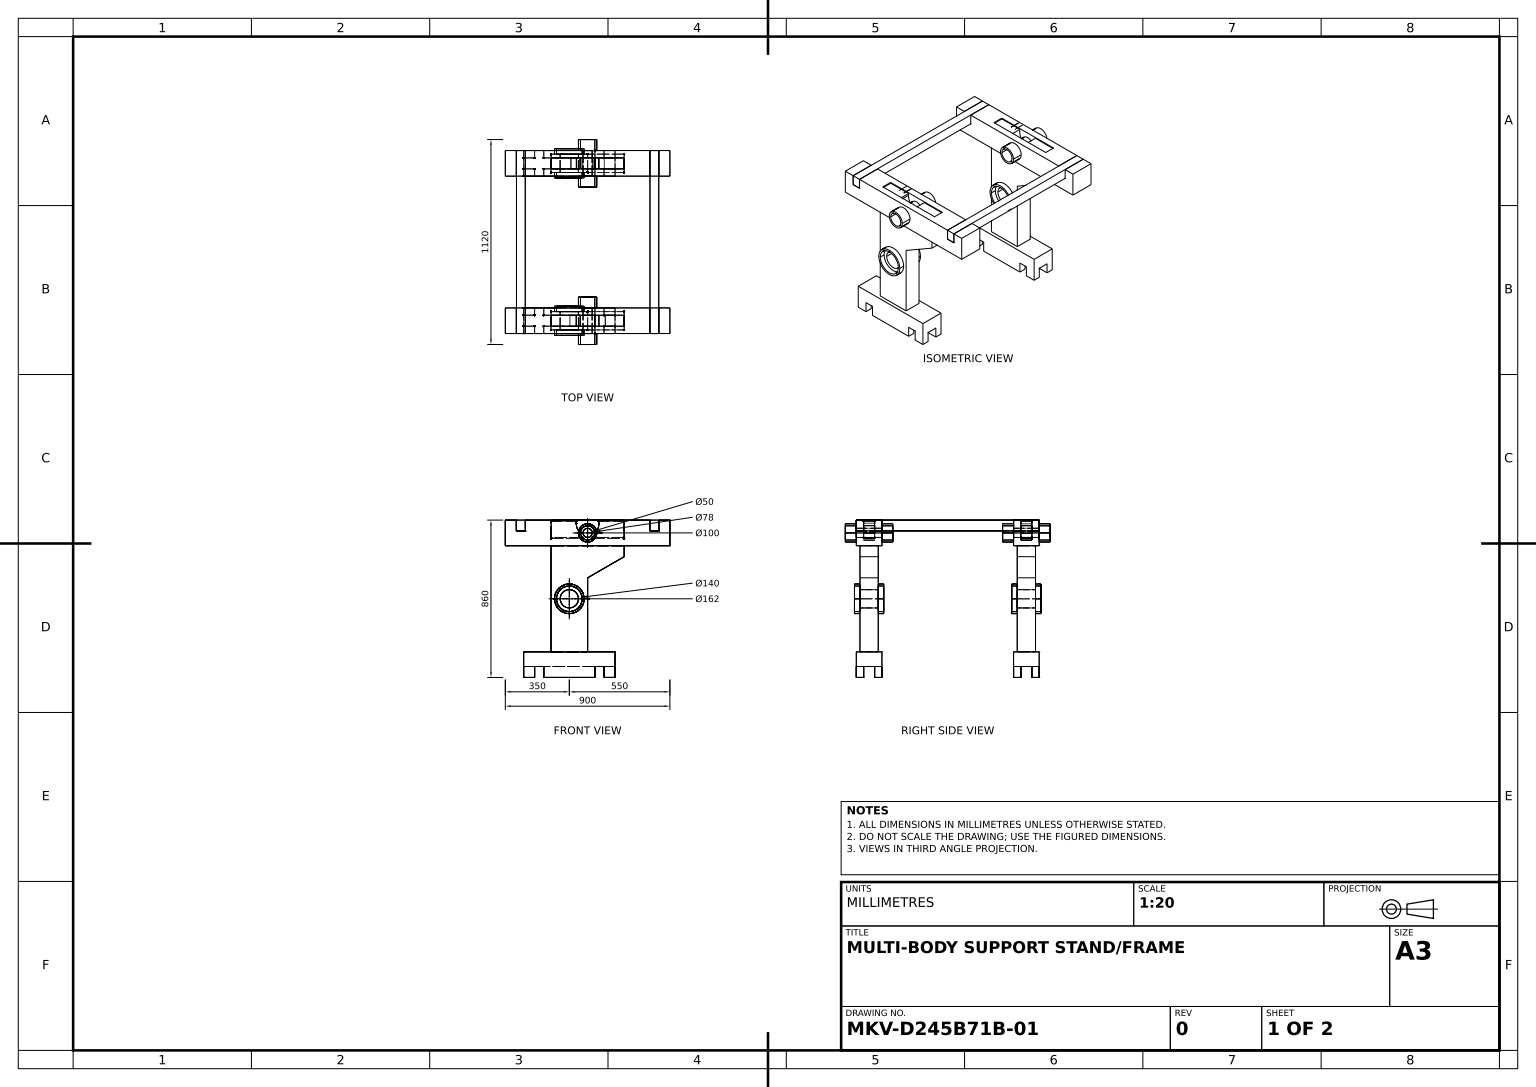
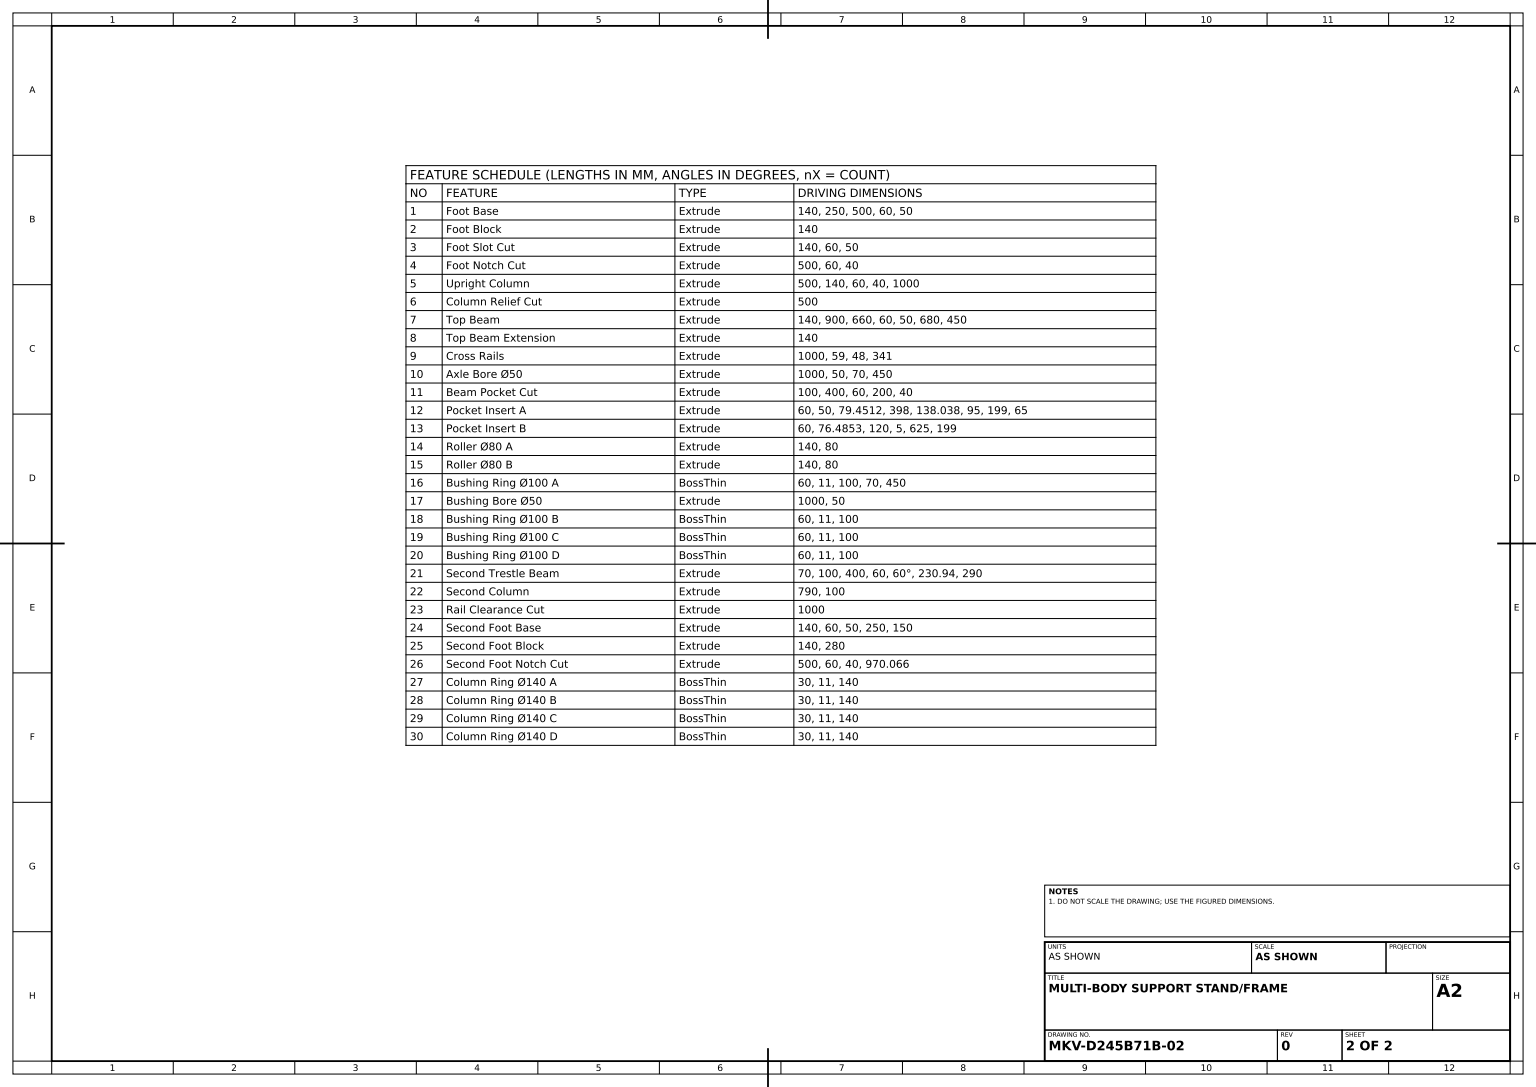
SolidWorks part; units mm, degrees
material "Plain Carbon Steel"
ref_plane "Front Plane" through (0, 0, 0) normal (0, 0, 1) x (1, 0, 0)
ref_plane "Top Plane" through (0, 0, 0) normal (0, 1, 0) x (1, 0, 0)
ref_plane "Right Plane" through (0, 0, 0) normal (1, 0, 0) x (0, 0, -1)
sketch "Foot Base Sketch" plane through (0, 0, 0) normal (0, 1, 0) x (1, 0, 0)
  line L0 (-250, 0) -> (-250, 140)
  line L1 (-250, 0) -> (250, 0)
  line L2 (-250, 140) -> (-190, 140)
  line L3 (-190, 140) -> (-190, 80)
  line L4 (-190, 80) -> (-140, 80)
  line L5 (-140, 80) -> (-140, 140)
  line L6 (-140, 140) -> (140, 140)
  line L7 (140, 140) -> (140, 80)
  line L8 (140, 80) -> (190, 80)
  line L9 (190, 80) -> (190, 140)
  line L10 (190, 140) -> (250, 140)
  line L11 (250, 140) -> (250, 0)
  dimension "D1" = 250
  dimension "D2" = 500
  dimension "D3" = 140
  dimension "D4" = 140
  dimension "D5" = 60
  dimension "D6" = 60
  dimension "D7" = 60
  dimension "D8" = 60
  dimension "D9" = 50
  dimension "D10" = 50
  dimension "D11" = 60
extrude "Foot Base" add sketch "Foot Base Sketch" along normal blind 140
sketch "Foot Block Sketch" plane through (0, 0, 0) normal (0, 0, 1) x (1, 0, 0)
  line L1 (-250, 140) -> (250, 140)
  line L2 (-250, 140) -> (-250, 0)
  line L3 (-250, 0) -> (250, 0)
  line L4 (250, 140) -> (250, 0)
extrude "Foot Block" add sketch "Foot Block Sketch" against normal blind 140
sketch "Foot Slot Sketch" plane through (0, 0, 0) normal (0, 0, 1) x (1, 0, 0)
  line L1 (-250, 0) -> (250, 0) construction
  line L2 (-190, 0) -> (-190, 60)
  line L3 (-190, 60) -> (-140, 60)
  line L4 (-140, 60) -> (-140, 0)
  line L6 (140, 0) -> (140, 60)
  line L7 (140, 60) -> (190, 60)
  line L8 (190, 60) -> (190, 0)
  line L13 (-190, 0) -> (-140, 0)
  line L14 (140, 0) -> (190, 0)
  line L15 (-250, 140) -> (-250, 0) construction
  line L16 (250, 140) -> (250, 0) construction
  point P17 (165, 60)
  dimension "D1" = 60
  dimension "D2" = 50
  dimension "D3" = 60
  dimension "D4" = 50
  dimension "D5" = 60
  dimension "D6" = 60
extrude "Foot Slot Cut" cut sketch "Foot Slot Sketch" against normal blind 140
sketch "Foot Notch Sketch" plane through (-250, 0, 0) normal (-1, 0, 0) x (0, 0, 1)
  line L0 (0, 140) -> (0, 0) construction
  line L3 (-140, 0) -> (0, 0) construction
  line L4 (-100, 0) -> (-100, 60)
  line L5 (-100, 60) -> (-40, 60)
  line L6 (-40, 60) -> (-40, 0)
  line L7 (-40, 0) -> (-100, 0)
  dimension "D1" = 60
  dimension "D2" = 60
  dimension "D3" = 40
extrude "Foot Notch Cut" cut sketch "Foot Notch Sketch" against normal blind 500
sketch "Upright Column Sketch" plane through (-250, 0, 0) normal (-1, 0, 0) x (0, 0, 1)
  line L0 (720, 140) -> (860, 140)
  line L1 (860, 140) -> (860, 0)
  line L2 (860, 0) -> (820, 0)
  line L3 (720, 0) -> (720, 140)
  line L4 (720, 0) -> (760, 0)
  line L5 (760, 0) -> (760, 60)
  line L6 (760, 60) -> (820, 60)
  line L7 (820, 60) -> (820, 0)
  line L8 (760, 0) -> (720, 0)
  line L9 (-140, 140) -> (-140, 0) construction
  dimension "D1" = 140
  dimension "D2" = 60
  dimension "D3" = 40
  dimension "D4" = 1000
  dimension "D5" = 60
extrude "Upright Column" add sketch "Upright Column Sketch" against normal blind 500 separate body contours L6 L7 L2 L1 L0 L3 L4 L5
sketch "Column Relief Sketch" plane through (0, 0, 720) normal (0, 0, -1) x (-1, 0, 0)
  line L0 (-190, 0) -> (-190, 60)
  line L1 (-190, 60) -> (-140, 60)
  line L2 (-190, 60) -> (-140, 60) construction
  line L3 (-140, 60) -> (-140, 0)
  line L4 (-140, 0) -> (-190, 0)
  line L5 (140, 60) -> (190, 60)
  line L6 (190, 60) -> (190, 0)
  line L7 (190, 0) -> (250, 0) construction
  line L8 (190, 60) -> (190, 0) construction
  line L9 (190, 0) -> (140, 0)
  line L10 (-140, 0) -> (140, 0) construction
  line L11 (-250, 0) -> (250, 0) construction
  line L12 (140, 0) -> (140, 60)
extrude "Column Relief Cut" cut sketch "Column Relief Sketch" against normal blind 500
sketch "Top Beam Sketch" plane through (0, 0, 860) normal (0, 0, 1) x (1, 0, 0)
  line L0 (-190, 60) -> (-140, 60) construction
  line L1 (450, 720) -> (-450, 720)
  line L2 (-450, 720) -> (-450, 860)
  line L3 (-450, 860) -> (-390, 860)
  line L4 (-390, 860) -> (-390, 800)
  line L5 (-390, 800) -> (-340, 800)
  line L6 (-340, 800) -> (-340, 860)
  line L9 (450, 720) -> (450, 860)
  line L10 (450, 860) -> (390, 860)
  line L11 (390, 860) -> (390, 800)
  line L12 (390, 800) -> (340, 800)
  line L13 (340, 800) -> (340, 860)
  line L14 (340, 860) -> (-340, 860)
  dimension "D1" = 900
  dimension "D2" = 660
  dimension "D3" = 140
  dimension "D4" = 60
  dimension "D5" = 50
  dimension "D6" = 60
  dimension "D7" = 680
  dimension "D8" = 140
  dimension "D9" = 60
  dimension "D10" = 60
  dimension "D11" = 60
  dimension "D12" = 450
extrude "Top Beam" add sketch "Top Beam Sketch" against normal blind 140 separate body
sketch "Top Beam Extension Sketch" plane through (0, 0, -140) normal (0, 0, -1) x (-1, 0, 0)
  line L0 (-450, 860) -> (-450, 720)
  line L1 (-450, 720) -> (450, 720)
  line L2 (450, 720) -> (450, 860)
  line L3 (450, 860) -> (390, 860)
  line L4 (390, 860) -> (390, 800)
  line L5 (390, 800) -> (340, 800)
  line L6 (340, 800) -> (340, 860)
  line L7 (340, 860) -> (-340, 860)
  line L8 (-340, 860) -> (-340, 800)
  line L9 (-340, 800) -> (-390, 800)
  line L10 (-390, 800) -> (-390, 860)
  line L11 (-390, 860) -> (-450, 860)
extrude "Top Beam Extension" add sketch "Top Beam Extension Sketch" against normal blind 140 separate body
sketch "Cross Rails Sketch" plane through (0, 0, 860) normal (0, 0, 1) x (1, 0, 0)
  line L1 (341, 860) -> (341, 801)
  line L3 (389, 860) -> (341, 860)
  line L4 (341, 801) -> (389, 801)
  line L5 (389, 801) -> (389, 860)
  line L7 (0, 860) -> (0, 140)
  line L8 (340, 860) -> (-340, 860) construction
  line L9 (250, 140) -> (-250, 140) construction
  line L10 (-389, 801) -> (-389, 860)
  line L11 (-341, 801) -> (-389, 801)
  line L12 (-341, 860) -> (-341, 801)
  line L13 (-389, 860) -> (-341, 860)
  dimension "D1" = 59
  dimension "D2" = 48
  dimension "D3" = 341
extrude "Cross Rails" add sketch "Cross Rails Sketch" against normal blind 1000 separate body contours L13 L10 L11 L12 | L4 L5 L3 L1
sketch "Axle Bore Ø50 Sketch" plane through (0, 0, 860) normal (0, 0, 1) x (1, 0, 0)
  line L0 (340, 860) -> (-340, 860) construction
  line L1 (450, 720) -> (450, 860) construction
  circle A0 centre (0, 790) radius 25
  dimension "D1" = 50
  dimension "D2" = 70
  dimension "D3" = 450
extrude "Axle Bore Ø50" cut sketch "Axle Bore Ø50 Sketch" against normal blind 1000
sketch "Beam Pocket Sketch" plane through (0, 860, 0) normal (0, 1, 0) x (1, 0, 0)
  line L0 (-389, -360) -> (389, -360)
  line L1 (340, -720) -> (-340, -720) construction
  line L2 (200, 40) -> (200, 100)
  line L3 (-200, -760) -> (200, -760)
  line L4 (-200, -760) -> (-200, -820)
  line L5 (-200, -820) -> (200, -820)
  line L6 (200, -760) -> (200, -820)
  line L7 (-389, 140) -> (-389, -860) construction
  line L8 (389, 140) -> (389, -860) construction
  line L9 (-200, 100) -> (200, 100)
  line L10 (-200, 40) -> (-200, 100)
  line L11 (-200, 40) -> (200, 40)
  dimension "D2" = 400
  dimension "D3" = 60
  dimension "D4" = 200
  dimension "D5" = 40
extrude "Beam Pocket Cut" cut sketch "Beam Pocket Sketch" against normal blind 100 contours L6 L3 L4 L5 | L10 L11 L2 L9
sketch "Pocket Insert A Sketch" plane through (0, 0, 760) normal (0, 0, 1) x (1, 0, 0)
  line L2 (-199, 855) -> (-199, 760)
  line L7 (199, 855) -> (199, 760)
  line L8 (199, 760) -> (-199, 760)
  line L9 (-199, 760) -> (-199, 855)
  line L10 (-199, 855) -> (-60.9618, 855)
  line L11 (60.9618, 855) -> (199, 855)
  circle A1 centre (0, 790) radius 25
  arc A2 (-60.9618, 855) -> (0, 765) centre (17.5, 842.5) ccw
  arc A3 (0, 765) -> (60.9618, 855) centre (-17.5, 842.5) ccw
  line M7 (-200, 760) -> (200, 760)
  circle M9 centre (0, 790) radius 25
  dimension "D1" = 79.4512
  dimension "D3" = 50
  dimension "D4" = 79.4512
  dimension "D2" = 138.0382
  dimension "D5" = 398
  dimension "D6" = 138.0382
  dimension "D7" = 95
  dimension "D8" = 199
  dimension "D9" = 65
extrude "Pocket Insert A" add sketch "Pocket Insert A Sketch" along normal blind 60 contours A3 A2 L10 L2 L7 L11 M9 M7
sketch "Pocket Insert B Sketch" plane through (0, 0, -40) normal (0, 0, -1) x (-1, 0, 0)
  line L0 (-199, 855) -> (-199, 765)
  line L1 (60, 855) -> (199, 855)
  line L3 (-199, 765) -> (199, 765)
  line L4 (199, 765) -> (199, 855)
  line L6 (-199, 855) -> (-60, 855)
  line L8 (340, 860) -> (-340, 860) construction
  line L9 (-250, 140) -> (250, 140) construction
  arc A1 (-60, 855) -> (0, 765) centre (15, 840) ccw
  arc A2 (60, 855) -> (0, 765) centre (-15, 840) cw
  circle M10 centre (0, 790) radius 25
  dimension "D1" = 76.4853
  dimension "D2" = 76.4853
  dimension "D3" = 120
  dimension "D4" = 5
  dimension "D5" = 199
  dimension "D6" = 199
  dimension "D7" = 60
  dimension "D8" = 625
extrude "Pocket Insert B" add sketch "Pocket Insert B Sketch" along normal blind 60 separate body contours A1 L6 L0 L3 M10 | L1 A2 L3 L4 M10
sketch "Roller Ø80 A Sketch" plane through (0, 0, 860) normal (0, 0, 1) x (1, 0, 0)
  circle A0 centre (0, 790) radius 40
  dimension "D1" = 80
extrude "Roller Ø80 A" add sketch "Roller Ø80 A Sketch" against normal blind 140
sketch "Roller Ø80 B Sketch" plane through (0, 0, -140) normal (0, 0, -1) x (-1, 0, 0)
  circle A0 centre (0, 790) radius 40
  dimension "D1" = 80
extrude "Roller Ø80 B" add sketch "Roller Ø80 B Sketch" against normal blind 140
sketch "Bushing Ring Ø100 A Sketch" plane through (0, 0, 860) normal (0, 0, 1) x (1, 0, 0)
  line L0 (340, 860) -> (-340, 860) construction
  line L1 (450, 720) -> (450, 860) construction
  circle A0 centre (0, 790) radius 50
  dimension "D1" = 100
  dimension "D2" = 70
  dimension "D3" = 450
extrude "Bushing Ring Ø100 A" add sketch "Bushing Ring Ø100 A Sketch" along normal blind 60 thin thin type one direction reverse wall 11
sketch "Bushing Bore Ø50 Sketch" plane through (0, 0, 860) normal (0, 0, 1) x (1, 0, 0)
  circle A0 centre (0, 790) radius 25
  dimension "D1" = 50
extrude "Bushing Bore Ø50" cut sketch "Bushing Bore Ø50 Sketch" against normal blind 1000
sketch "Bushing Ring Ø100 B Sketch" plane through (0, 0, 720) normal (0, 0, -1) x (-1, 0, 0)
  circle A0 centre (0, 790) radius 50
  dimension "D1" = 100
extrude "Bushing Ring Ø100 B" add sketch "Bushing Ring Ø100 B Sketch" along normal blind 60 thin thin type one direction reverse wall 11
sketch "Bushing Ring Ø100 C Sketch" plane through (0, 0, 0) normal (0, 0, 1) x (1, 0, 0)
  circle A0 centre (0, 790) radius 50
  dimension "D1" = 100
extrude "Bushing Ring Ø100 C" add sketch "Bushing Ring Ø100 C Sketch" along normal blind 60 thin thin type one direction reverse wall 11
sketch "Bushing Ring Ø100 D Sketch" plane through (0, 0, -140) normal (0, 0, -1) x (-1, 0, 0)
  circle A0 centre (0, 790) radius 50
  dimension "D1" = 100
extrude "Bushing Ring Ø100 D" add sketch "Bushing Ring Ø100 D Sketch" along normal blind 60 thin thin type one direction reverse wall 11
ref_plane "Plane1" through (0, 0, -70) normal (0, 0, 1) x (1, 0, 0)
sketch "Second Trestle Beam Sketch" plane through (0, 0, -70) normal (0, 0, 1) x (1, 0, 0)
  line L0 (200, 720) -> (-200, 720)
  line L1 (450, 720) -> (-450, 720) construction
  line L2 (200, 720) -> (200, 660)
  line L3 (200, 720) -> (200, 660)
  line L4 (200, 660) -> (0, 544.5299)
  line L7 (250, 140) -> (-250, 140) construction
  line L8 (-200, 720) -> (-200, 140)
  line L9 (-200, 140) -> (0, 140)
  line L10 (0, 140) -> (0, 544.5299)
  circle A0 centre (-100, 430) radius 50
  point P5 (0, 720)
  point P13 (0, 140)
  dimension "D5" = 100
  dimension "D1" = 400
  dimension "D2" = 60
  dimension "D3" = 60
  dimension "D4" = 230.9401
  dimension "D6" = 100
  dimension "D7" = 290
extrude "Second Trestle Beam" add sketch "Second Trestle Beam Sketch" along normal mid plane 100 contours L9 L10 L4 L2 L0 L8 A0
ref_plane "Plane3" through (0, 0, 790) normal (0, 0, 1) x (1, 0, 0)
sketch "Second Column Sketch" plane through (0, 0, 790) normal (0, 0, 1) x (1, 0, 0)
  line L0 (-200, 720) -> (200, 720)
  line L1 (200, 720) -> (200, 660)
  line L2 (200, 660) -> (0, 544.5299)
  line L3 (0, 544.5299) -> (0, 140)
  line L4 (250, 140) -> (-250, 140) construction
  line L5 (0, 140) -> (-200, 140)
  line L6 (-200, 140) -> (0, 140) construction
  line L7 (-200, 140) -> (-200, 720)
  circle A0 centre (-100, 430) radius 50
  dimension "D1" = 100
extrude "Second Column" add sketch "Second Column Sketch" along normal mid plane 100
sketch "Rail Clearance Sketch" plane through (0, 0, 860) normal (0, 0, 1) x (1, 0, 0)
  line L1 (-250, 140) -> (250, 140)
  line L2 (-250, 140) -> (-250, 0)
  line L3 (-250, 0) -> (250, 0)
  line L4 (250, 140) -> (250, 0)
extrude "Rail Clearance Cut" cut sketch "Rail Clearance Sketch" against normal blind 1000
sketch "Second Foot Base Sketch" plane through (0, 0, 860) normal (0, 0, 1) x (1, 0, 0)
  line L0 (-350, 140) -> (-350, 0)
  line L2 (-350, 140) -> (150, 140)
  line L3 (-350, 0) -> (-290, 0)
  line L4 (-290, 0) -> (-290, 60)
  line L5 (-290, 60) -> (-240, 60)
  line L6 (-240, 60) -> (-240, 0)
  line L7 (-240, 0) -> (40, 0)
  line L8 (40, 0) -> (40, 60)
  line L9 (40, 60) -> (90, 60)
  line L10 (90, 60) -> (90, 0)
  line L11 (90, 0) -> (150, 0)
  line L12 (150, 0) -> (150, 140)
  line L14 (340, 860) -> (-340, 860) construction
  point P12 (-100, 140)
  point P17 (0, 860)
  dimension "D1" = 140
  dimension "D2" = 60
  dimension "D3" = 60
  dimension "D4" = 50
  dimension "D5" = 50
  dimension "D6" = 60
  dimension "D7" = 60
  dimension "D8" = 250
  dimension "D9" = 150
extrude "Second Foot Base" add sketch "Second Foot Base Sketch" against normal blind 140
sketch "Second Foot Block Sketch" plane through (0, 0, -140) normal (0, 0, -1) x (-1, 0, 0)
  line L0 (-150, 140) -> (350, 140)
  line L1 (350, 140) -> (350, 0)
  line L2 (350, 0) -> (290, 0)
  line L3 (290, 0) -> (290, 60)
  line L4 (290, 60) -> (240, 60)
  line L5 (240, 60) -> (240, 0)
  line L6 (240, 0) -> (-40, 0)
  line L7 (240, 0) -> (-40, 0) construction
  line L8 (-40, 0) -> (-40, 60)
  line L9 (-40, 60) -> (-90, 60)
  line L10 (-90, 60) -> (-90, 0)
  line L11 (-90, 0) -> (-150, 0) construction
  line L12 (-90, 0) -> (-150, 0)
  line L13 (-150, 0) -> (-150, 140)
  dimension "D1" = 280
extrude "Second Foot Block" add sketch "Second Foot Block Sketch" against normal blind 140
sketch "Second Foot Notch Sketch" plane through (-350, 0, 0) normal (-1, 0, 0) x (0, 0, 1)
  line L0 (-140, 0) -> (-140, 140) construction
  line L1 (0, 0) -> (-140, 0) construction
  line L2 (-100, 0) -> (-100, 60)
  line L3 (-100, 60) -> (-40, 60)
  line L4 (-40, 60) -> (-40, 0)
  line L5 (-40, 0) -> (-100, 0)
  line L6 (360, 860) -> (360, -110.0657)
  line L7 (-140, 860) -> (860, 860) construction
  line L8 (760, 60) -> (760, 0)
  line L9 (760, 0) -> (820, 0)
  line L10 (820, 0) -> (820, 60)
  line L11 (820, 60) -> (760, 60)
  line M7 (-140, 0) -> (0, 0)
  dimension "D1" = 60
  dimension "D2" = 60
  dimension "D3" = 40
  dimension "D4" = 970.0657
extrude "Second Foot Notch Cut" cut sketch "Second Foot Notch Sketch" against normal blind 500 contours L4 L3 L2 M7 | L10 L11 L8 L9
sketch "Column Ring Ø140 A Sketch" plane through (0, 0, 840) normal (0, 0, 1) x (1, 0, 0)
  circle A0 centre (-100, 430) radius 70
  dimension "D1" = 140
extrude "Column Ring Ø140 A" add sketch "Column Ring Ø140 A Sketch" along normal blind 30 thin
sketch "Column Ring Ø140 B Sketch" plane through (0, 0, 740) normal (0, 0, -1) x (-1, 0, 0)
  circle A0 centre (100, 430) radius 70
  dimension "D1" = 140
extrude "Column Ring Ø140 B" add sketch "Column Ring Ø140 B Sketch" along normal blind 30 thin
sketch "Column Ring Ø140 C Sketch" plane through (0, 0, -20) normal (0, 0, 1) x (1, 0, 0)
  circle A0 centre (-100, 430) radius 70
  dimension "D1" = 140
extrude "Column Ring Ø140 C" add sketch "Column Ring Ø140 C Sketch" along normal blind 30 thin
sketch "Column Ring Ø140 D Sketch" plane through (0, 0, -120) normal (0, 0, -1) x (-1, 0, 0)
  circle A0 centre (100, 430) radius 70
  dimension "D1" = 140
extrude "Column Ring Ø140 D" add sketch "Column Ring Ø140 D Sketch" along normal blind 30 thin
